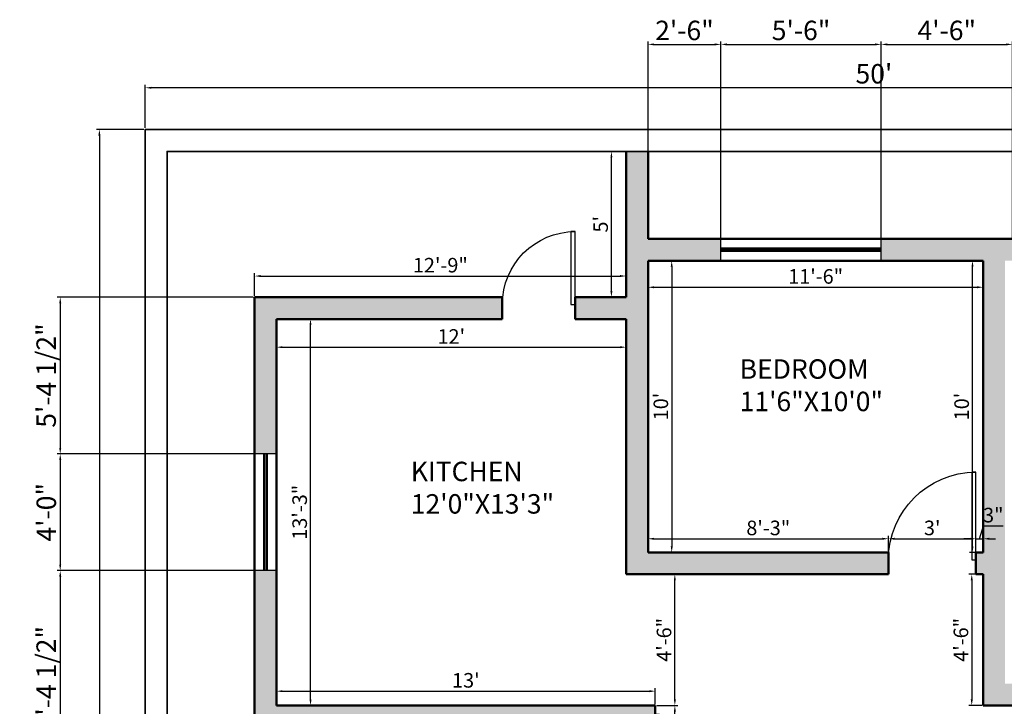
# Model space of a CAD drawing. Units: inches. Extents: x 2442 to 3851, y 589 to 2836.
# Tile 15 of 22: x 2442 to 2847, y 2554 to 2836. Entities that reach past the tile are written whole.
import ezdxf

# ---------------------------------------------------------------- set-up
doc = ezdxf.new("R2010")
doc.units = ezdxf.units.IN
for name, color, linetype, lineweight in [('A-ANNO-DIMS', 2, 'Continuous', 18), ('A-AREA-IDEN', 7, 'Continuous', 18), ('A-DOOR', 4, 'Continuous', 25), ('A-GLAZ', 1, 'Continuous', 25), ('A-WALL', 7, 'Continuous', 50), ('A-WALL-PATT', 8, 'Continuous', 13), ('C-PROP', 7, 'Continuous', 35)]:
    doc.layers.add(name, color=color, linetype=linetype, lineweight=lineweight)
doc.styles.get("Standard").update_dxf_attribs({"font": 'arial.ttf'})
doc.dimstyles.new('ISO-25', dxfattribs={"dimtxt": 8, "dimasz": 2.5, "dimexe": 1.25, "dimexo": 0.625, "dimtad": 1, "dimlunit": 3, "dimtxsty": 'Standard', "dimcen": 2.5, "dimadec": 0, "dimazin": 0, "dimtfac": 1, "dimtmove": 0, "dimatfit": 3, "dimfxl": 1, "dimarcsym": 0})

# ---------------------------------------------------------------- blocks, each defined once
blk = doc.blocks.new('*U23')
for p, q in [((0, 0), (0, -6)), ((36, 0), (36, -6))]:
    blk.add_line(p, q)
blk.add_lwpolyline([(0, 0), (0, 36), (1.75, 36), (1.75, 0)], close=True)
blk.add_arc((0, 0), 36, 0, 90)
blk = doc.blocks.new('*U24')
for p, q in [((0, 0), (0, -6)), ((30, 0), (30, -6))]:
    blk.add_line(p, q)
blk.add_lwpolyline([(0, 0), (0, 30), (1.75, 30), (1.75, 0)], close=True)
blk.add_arc((0, 0), 30, 0, 90)
blk = doc.blocks.new('*D35')
at = {"layer": 'A-ANNO-DIMS', "color": 0, "lineweight": -2, "transparency": 16777216}
for p, q in [((2493.6, 2791.83), (2493.6, 2809.62)), ((3093.6, 2791.83), (3093.6, 2809.62)), ((3091.1, 2808.37), (2496.1, 2808.37))]:
    blk.add_line(p, q, dxfattribs=at)
at = {"layer": 'A-ANNO-DIMS', "color": 0, "transparency": 16777216}
for points in [[(2496.1, 2808.78), (2496.1, 2807.95), (2493.6, 2808.37)], [(3091.1, 2808.78), (3091.1, 2807.95), (3093.6, 2808.37)]]:
    blk.add_solid(points, dxfattribs=at)
at = {"layer": 'Defpoints', "color": 0, "transparency": 16777216}
for p in [(2493.6, 2808.37), (2493.6, 2791.21), (3093.6, 2791.21)]:
    blk.add_point(p, dxfattribs=at)
at = {"layer": 'A-ANNO-DIMS', "color": 0, "transparency": 16777216, "insert": (2793.6, 2813.08), "char_height": 8, "attachment_point": 5}
blk.add_mtext("50'", dxfattribs=at)
blk = doc.blocks.new('*D36')
at = {"layer": 'A-ANNO-DIMS', "color": 0, "lineweight": -2, "transparency": 16777216}
for p, q in [((2492.97, 2791.21), (2473.47, 2791.21)), ((2474.72, 2788.71), (2474.72, 2193.71)), ((2492.97, 2191.21), (2473.47, 2191.21))]:
    blk.add_line(p, q, dxfattribs=at)
at = {"layer": 'A-ANNO-DIMS', "color": 0, "transparency": 16777216}
for points in [[(2474.3, 2788.71), (2475.14, 2788.71), (2474.72, 2791.21)], [(2474.3, 2193.71), (2475.14, 2193.71), (2474.72, 2191.21)]]:
    blk.add_solid(points, dxfattribs=at)
at = {"layer": 'Defpoints', "color": 0, "transparency": 16777216}
for p in [(2493.6, 2791.21), (2474.72, 2191.21), (2493.6, 2191.21)]:
    blk.add_point(p, dxfattribs=at)
at = {"layer": 'A-ANNO-DIMS', "color": 0, "transparency": 16777216, "insert": (2470.01, 2491.21), "char_height": 8, "attachment_point": 5, "rotation": 90}
blk.add_mtext("50'", dxfattribs=at)
blk = doc.blocks.new('*D37')
at = {"layer": 'A-ANNO-DIMS', "color": 0, "lineweight": -2, "transparency": 16777216}
for p, q in [((2548.22, 2713.21), (2562.89, 2713.21)), ((2561.64, 2556.71), (2561.64, 2710.71)), ((2548.22, 2554.21), (2562.89, 2554.21))]:
    blk.add_line(p, q, dxfattribs=at)
at = {"layer": 'A-ANNO-DIMS', "color": 0, "transparency": 16777216}
for points in [[(2561.22, 2710.71), (2562.05, 2710.71), (2561.64, 2713.21)], [(2561.22, 2556.71), (2562.05, 2556.71), (2561.64, 2554.21)]]:
    blk.add_solid(points, dxfattribs=at)
at = {"layer": 'Defpoints', "color": 0, "transparency": 16777216}
for p in [(2547.6, 2713.21), (2561.64, 2713.21), (2547.6, 2554.21)]:
    blk.add_point(p, dxfattribs=at)
at = {"layer": 'A-ANNO-DIMS', "color": 0, "transparency": 16777216, "insert": (2557.95, 2633.71), "char_height": 6, "attachment_point": 5, "rotation": 90}
blk.add_mtext('13\'-3"', dxfattribs=at)
blk = doc.blocks.new('*D38')
at = {"layer": 'A-ANNO-DIMS', "color": 0, "lineweight": -2, "transparency": 16777216}
for p, q in [((2547.6, 2712.58), (2547.6, 2700.38)), ((2691.6, 2712.58), (2691.6, 2700.38)), ((2550.1, 2701.63), (2689.1, 2701.63))]:
    blk.add_line(p, q, dxfattribs=at)
at = {"layer": 'A-ANNO-DIMS', "color": 0, "transparency": 16777216}
for points in [[(2550.1, 2702.05), (2550.1, 2701.22), (2547.6, 2701.63)], [(2689.1, 2702.05), (2689.1, 2701.22), (2691.6, 2701.63)]]:
    blk.add_solid(points, dxfattribs=at)
at = {"layer": 'Defpoints', "color": 0, "transparency": 16777216}
for p in [(2547.6, 2713.21), (2691.6, 2713.21), (2691.6, 2701.63)]:
    blk.add_point(p, dxfattribs=at)
at = {"layer": 'A-ANNO-DIMS', "color": 0, "transparency": 16777216, "insert": (2619.6, 2705.27), "char_height": 6, "attachment_point": 5}
blk.add_mtext("12'", dxfattribs=at)
blk = doc.blocks.new('*D39')
at = {"layer": 'A-ANNO-DIMS', "color": 0, "lineweight": -2, "transparency": 16777216}
for p, q in [((2690.97, 2782.21), (2684.27, 2782.21)), ((2685.52, 2724.71), (2685.52, 2779.71)), ((2690.97, 2722.21), (2684.27, 2722.21))]:
    blk.add_line(p, q, dxfattribs=at)
at = {"layer": 'A-ANNO-DIMS', "color": 0, "transparency": 16777216}
for points in [[(2685.11, 2779.71), (2685.94, 2779.71), (2685.52, 2782.21)], [(2685.11, 2724.71), (2685.94, 2724.71), (2685.52, 2722.21)]]:
    blk.add_solid(points, dxfattribs=at)
at = {"layer": 'Defpoints', "color": 0, "transparency": 16777216}
for p in [(2685.52, 2782.21), (2691.6, 2782.21), (2691.6, 2722.21)]:
    blk.add_point(p, dxfattribs=at)
at = {"layer": 'A-ANNO-DIMS', "color": 0, "transparency": 16777216, "insert": (2681.85, 2752.21), "char_height": 6, "attachment_point": 5, "rotation": 90}
blk.add_mtext("5'", dxfattribs=at)
blk = doc.blocks.new('*D40')
at = {"layer": 'A-ANNO-DIMS', "color": 0, "lineweight": -2, "transparency": 16777216}
for p, q in [((2538.6, 2722.83), (2538.6, 2732.15)), ((2541.1, 2730.9), (2689.1, 2730.9)), ((2691.6, 2722.83), (2691.6, 2732.15))]:
    blk.add_line(p, q, dxfattribs=at)
at = {"layer": 'A-ANNO-DIMS', "color": 0, "transparency": 16777216}
for points in [[(2541.1, 2731.32), (2541.1, 2730.49), (2538.6, 2730.9)], [(2689.1, 2731.32), (2689.1, 2730.49), (2691.6, 2730.9)]]:
    blk.add_solid(points, dxfattribs=at)
at = {"layer": 'Defpoints', "color": 0, "transparency": 16777216}
for p in [(2691.6, 2730.9), (2538.6, 2722.21), (2691.6, 2722.21)]:
    blk.add_point(p, dxfattribs=at)
at = {"layer": 'A-ANNO-DIMS', "color": 0, "transparency": 16777216, "insert": (2615.1, 2734.59), "char_height": 6, "attachment_point": 5}
blk.add_mtext('12\'-9"', dxfattribs=at)
blk = doc.blocks.new('*D44')
at = {"layer": 'A-ANNO-DIMS', "color": 0, "lineweight": -2, "transparency": 16777216}
for p, q in [((2700.6, 2736.58), (2700.6, 2725.04)), ((2838.6, 2736.58), (2838.6, 2725.04)), ((2703.1, 2726.29), (2836.1, 2726.29))]:
    blk.add_line(p, q, dxfattribs=at)
at = {"layer": 'A-ANNO-DIMS', "color": 0, "transparency": 16777216}
for points in [[(2703.1, 2726.7), (2703.1, 2725.87), (2700.6, 2726.29)], [(2836.1, 2726.7), (2836.1, 2725.87), (2838.6, 2726.29)]]:
    blk.add_solid(points, dxfattribs=at)
at = {"layer": 'Defpoints', "color": 0, "transparency": 16777216}
for p in [(2700.6, 2737.21), (2838.6, 2737.21), (2838.6, 2726.29)]:
    blk.add_point(p, dxfattribs=at)
at = {"layer": 'A-ANNO-DIMS', "color": 0, "transparency": 16777216, "insert": (2769.6, 2729.98), "char_height": 6, "attachment_point": 5}
blk.add_mtext('11\'-6"', dxfattribs=at)
blk = doc.blocks.new('*D45')
at = {"layer": 'A-ANNO-DIMS', "color": 0, "lineweight": -2, "transparency": 16777216}
for p, q in [((2701.22, 2737.21), (2711.59, 2737.21)), ((2710.34, 2734.71), (2710.34, 2619.71)), ((2701.22, 2617.21), (2711.59, 2617.21))]:
    blk.add_line(p, q, dxfattribs=at)
at = {"layer": 'A-ANNO-DIMS', "color": 0, "transparency": 16777216}
for points in [[(2709.93, 2734.71), (2710.76, 2734.71), (2710.34, 2737.21)], [(2709.93, 2619.71), (2710.76, 2619.71), (2710.34, 2617.21)]]:
    blk.add_solid(points, dxfattribs=at)
at = {"layer": 'Defpoints', "color": 0, "transparency": 16777216}
for p in [(2700.6, 2737.21), (2700.6, 2617.21), (2710.34, 2617.21)]:
    blk.add_point(p, dxfattribs=at)
at = {"layer": 'A-ANNO-DIMS', "color": 0, "transparency": 16777216, "insert": (2706.65, 2677.21), "char_height": 6, "attachment_point": 5, "rotation": 90}
blk.add_mtext("10'", dxfattribs=at)
blk = doc.blocks.new('*D60')
at = {"layer": 'A-ANNO-DIMS', "color": 0, "lineweight": -2, "transparency": 16777216}
for p, q in [((2837.97, 2737.21), (2832.93, 2737.21)), ((2834.18, 2619.71), (2834.18, 2734.71)), ((2837.97, 2617.21), (2832.93, 2617.21))]:
    blk.add_line(p, q, dxfattribs=at)
at = {"layer": 'A-ANNO-DIMS', "color": 0, "transparency": 16777216}
for points in [[(2833.76, 2734.71), (2834.6, 2734.71), (2834.18, 2737.21)], [(2833.76, 2619.71), (2834.6, 2619.71), (2834.18, 2617.21)]]:
    blk.add_solid(points, dxfattribs=at)
at = {"layer": 'Defpoints', "color": 0, "transparency": 16777216}
for p in [(2834.18, 2737.21), (2838.6, 2737.21), (2838.6, 2617.21)]:
    blk.add_point(p, dxfattribs=at)
at = {"layer": 'A-ANNO-DIMS', "color": 0, "transparency": 16777216, "insert": (2830.49, 2677.21), "char_height": 6, "attachment_point": 5, "rotation": 90}
blk.add_mtext("10'", dxfattribs=at)
blk = doc.blocks.new('*D61')
at = {"layer": 'A-ANNO-DIMS', "color": 0, "lineweight": -2, "transparency": 16777216}
for p, q in [((2700.6, 2617.83), (2700.6, 2624.06)), ((2703.1, 2622.81), (2797.1, 2622.81)), ((2799.6, 2617.83), (2799.6, 2624.06))]:
    blk.add_line(p, q, dxfattribs=at)
at = {"layer": 'A-ANNO-DIMS', "color": 0, "transparency": 16777216}
for points in [[(2703.1, 2623.23), (2703.1, 2622.4), (2700.6, 2622.81)], [(2797.1, 2623.23), (2797.1, 2622.4), (2799.6, 2622.81)]]:
    blk.add_solid(points, dxfattribs=at)
at = {"layer": 'Defpoints', "color": 0, "transparency": 16777216}
for p in [(2799.6, 2622.81), (2700.6, 2617.21), (2799.6, 2617.21)]:
    blk.add_point(p, dxfattribs=at)
at = {"layer": 'A-ANNO-DIMS', "color": 0, "transparency": 16777216, "insert": (2750.1, 2626.5), "char_height": 6, "attachment_point": 5}
blk.add_mtext('8\'-3"', dxfattribs=at)
blk = doc.blocks.new('*D62')
at = {"layer": 'A-ANNO-DIMS', "color": 0, "lineweight": -2, "transparency": 16777216}
for p, q in [((2799.6, 2617.83), (2799.6, 2624.06)), ((2802.1, 2622.81), (2833.1, 2622.81)), ((2835.6, 2614.83), (2835.6, 2624.06))]:
    blk.add_line(p, q, dxfattribs=at)
at = {"layer": 'A-ANNO-DIMS', "color": 0, "transparency": 16777216}
for points in [[(2802.1, 2623.23), (2802.1, 2622.4), (2799.6, 2622.81)], [(2833.1, 2623.23), (2833.1, 2622.4), (2835.6, 2622.81)]]:
    blk.add_solid(points, dxfattribs=at)
at = {"layer": 'Defpoints', "color": 0, "transparency": 16777216}
for p in [(2835.6, 2622.81), (2799.6, 2617.21), (2835.6, 2614.21)]:
    blk.add_point(p, dxfattribs=at)
at = {"layer": 'A-ANNO-DIMS', "color": 0, "transparency": 16777216, "insert": (2817.6, 2626.5), "char_height": 6, "attachment_point": 5}
blk.add_mtext("3'", dxfattribs=at)
blk = doc.blocks.new('*D63')
at = {"layer": 'A-ANNO-DIMS', "color": 0, "lineweight": -2, "transparency": 16777216}
for p, q in [((2837.1, 2622.81), (2838.67, 2628.07)), ((2838.67, 2628.07), (2846.82, 2628.07)), ((2833.1, 2622.81), (2830.6, 2622.81)), ((2835.6, 2614.83), (2835.6, 2624.06)), ((2835.6, 2622.81), (2838.6, 2622.81)), ((2835.6, 2622.81), (2838.6, 2622.81)), ((2838.6, 2617.83), (2838.6, 2624.06)), ((2841.1, 2622.81), (2843.6, 2622.81))]:
    blk.add_line(p, q, dxfattribs=at)
at = {"layer": 'A-ANNO-DIMS', "color": 0, "transparency": 16777216}
for points in [[(2833.1, 2623.23), (2833.1, 2622.4), (2835.6, 2622.81)], [(2841.1, 2623.23), (2841.1, 2622.4), (2838.6, 2622.81)]]:
    blk.add_solid(points, dxfattribs=at)
at = {"layer": 'Defpoints', "color": 0, "transparency": 16777216}
for p in [(2838.6, 2622.81), (2838.6, 2617.21), (2835.6, 2614.21)]:
    blk.add_point(p, dxfattribs=at)
at = {"layer": 'A-ANNO-DIMS', "color": 0, "transparency": 16777216, "insert": (2842.75, 2631.76), "char_height": 6, "attachment_point": 5}
blk.add_mtext('3"', dxfattribs=at)
blk = doc.blocks.new('*D85')
at = {"layer": 'A-ANNO-DIMS', "color": 0, "lineweight": -2, "transparency": 16777216}
for p, q in [((2704.22, 2554.21), (2712.89, 2554.21)), ((2711.64, 2544.71), (2711.64, 2551.71)), ((2704.22, 2542.21), (2712.89, 2542.21))]:
    blk.add_line(p, q, dxfattribs=at)
at = {"layer": 'A-ANNO-DIMS', "color": 0, "transparency": 16777216}
for points in [[(2711.22, 2551.71), (2712.05, 2551.71), (2711.64, 2554.21)], [(2711.22, 2544.71), (2712.05, 2544.71), (2711.64, 2542.21)]]:
    blk.add_solid(points, dxfattribs=at)
at = {"layer": 'Defpoints', "color": 0, "transparency": 16777216}
for p in [(2703.6, 2554.21), (2711.64, 2554.21), (2703.6, 2542.21)]:
    blk.add_point(p, dxfattribs=at)
at = {"layer": 'A-ANNO-DIMS', "color": 0, "transparency": 16777216, "insert": (2708, 2548.21), "char_height": 6, "attachment_point": 5, "rotation": 90}
blk.add_mtext("1'", dxfattribs=at)
blk = doc.blocks.new('*D86')
at = {"layer": 'A-ANNO-DIMS', "color": 0, "lineweight": -2, "transparency": 16777216}
for p, q in [((2709.79, 2608.21), (2712.89, 2608.21)), ((2711.64, 2556.71), (2711.64, 2605.71)), ((2704.22, 2554.21), (2712.89, 2554.21))]:
    blk.add_line(p, q, dxfattribs=at)
at = {"layer": 'A-ANNO-DIMS', "color": 0, "transparency": 16777216}
for points in [[(2711.22, 2605.71), (2712.05, 2605.71), (2711.64, 2608.21)], [(2711.22, 2556.71), (2712.05, 2556.71), (2711.64, 2554.21)]]:
    blk.add_solid(points, dxfattribs=at)
at = {"layer": 'Defpoints', "color": 0, "transparency": 16777216}
for p in [(2709.17, 2608.21), (2711.64, 2608.21), (2703.6, 2554.21)]:
    blk.add_point(p, dxfattribs=at)
at = {"layer": 'A-ANNO-DIMS', "color": 0, "transparency": 16777216, "insert": (2707.95, 2581.21), "char_height": 6, "attachment_point": 5, "rotation": 90}
blk.add_mtext('4\'-6"', dxfattribs=at)
blk = doc.blocks.new('*D87')
at = {"layer": 'A-ANNO-DIMS', "color": 0, "lineweight": -2, "transparency": 16777216}
for p, q in [((2837.97, 2608.21), (2832.63, 2608.21)), ((2833.88, 2605.71), (2833.88, 2556.71)), ((2837.97, 2554.21), (2832.63, 2554.21))]:
    blk.add_line(p, q, dxfattribs=at)
at = {"layer": 'A-ANNO-DIMS', "color": 0, "transparency": 16777216}
for points in [[(2833.46, 2605.71), (2834.29, 2605.71), (2833.88, 2608.21)], [(2833.46, 2556.71), (2834.29, 2556.71), (2833.88, 2554.21)]]:
    blk.add_solid(points, dxfattribs=at)
at = {"layer": 'Defpoints', "color": 0, "transparency": 16777216}
for p in [(2838.6, 2608.21), (2833.88, 2554.21), (2838.6, 2554.21)]:
    blk.add_point(p, dxfattribs=at)
at = {"layer": 'A-ANNO-DIMS', "color": 0, "transparency": 16777216, "insert": (2830.19, 2581.21), "char_height": 6, "attachment_point": 5, "rotation": 90}
blk.add_mtext('4\'-6"', dxfattribs=at)
blk = doc.blocks.new('*D88')
at = {"layer": 'A-ANNO-DIMS', "color": 0, "lineweight": -2, "transparency": 16777216}
for p, q in [((2547.6, 2554.83), (2547.6, 2561.35)), ((2550.1, 2560.1), (2701.1, 2560.1)), ((2703.6, 2554.83), (2703.6, 2561.35))]:
    blk.add_line(p, q, dxfattribs=at)
at = {"layer": 'A-ANNO-DIMS', "color": 0, "transparency": 16777216}
for points in [[(2550.1, 2560.52), (2550.1, 2559.68), (2547.6, 2560.1)], [(2701.1, 2560.52), (2701.1, 2559.68), (2703.6, 2560.1)]]:
    blk.add_solid(points, dxfattribs=at)
at = {"layer": 'Defpoints', "color": 0, "transparency": 16777216}
for p in [(2703.6, 2560.1), (2547.6, 2554.21), (2703.6, 2554.21)]:
    blk.add_point(p, dxfattribs=at)
at = {"layer": 'A-ANNO-DIMS', "color": 0, "transparency": 16777216, "insert": (2625.6, 2563.79), "char_height": 6, "attachment_point": 5}
blk.add_mtext("13'", dxfattribs=at)
blk = doc.blocks.new('*D182')
at = {"layer": 'A-ANNO-DIMS', "color": 0, "lineweight": -2, "transparency": 16777216}
for p, q in [((2700.6, 2746.83), (2700.6, 2827.46)), ((2703.1, 2826.21), (2728.1, 2826.21)), ((2730.6, 2746.83), (2730.6, 2827.46))]:
    blk.add_line(p, q, dxfattribs=at)
at = {"layer": 'A-ANNO-DIMS', "color": 0, "transparency": 16777216}
for points in [[(2703.1, 2826.62), (2703.1, 2825.79), (2700.6, 2826.21)], [(2728.1, 2826.62), (2728.1, 2825.79), (2730.6, 2826.21)]]:
    blk.add_solid(points, dxfattribs=at)
at = {"layer": 'Defpoints', "color": 0, "transparency": 16777216}
for p in [(2730.6, 2826.21), (2700.6, 2746.21), (2730.6, 2746.21)]:
    blk.add_point(p, dxfattribs=at)
at = {"layer": 'A-ANNO-DIMS', "color": 0, "transparency": 16777216, "insert": (2715.6, 2830.92), "char_height": 8, "attachment_point": 5}
blk.add_mtext('2\'-6"', dxfattribs=at)
blk = doc.blocks.new('*D183')
at = {"layer": 'A-ANNO-DIMS', "color": 0, "lineweight": -2, "transparency": 16777216}
for p, q in [((2730.6, 2746.83), (2730.6, 2827.46)), ((2733.1, 2826.21), (2794.1, 2826.21)), ((2796.6, 2746.83), (2796.6, 2827.46))]:
    blk.add_line(p, q, dxfattribs=at)
at = {"layer": 'A-ANNO-DIMS', "color": 0, "transparency": 16777216}
for points in [[(2733.1, 2826.62), (2733.1, 2825.79), (2730.6, 2826.21)], [(2794.1, 2826.62), (2794.1, 2825.79), (2796.6, 2826.21)]]:
    blk.add_solid(points, dxfattribs=at)
at = {"layer": 'Defpoints', "color": 0, "transparency": 16777216}
for p in [(2796.6, 2826.21), (2730.6, 2746.21), (2796.6, 2746.21)]:
    blk.add_point(p, dxfattribs=at)
at = {"layer": 'A-ANNO-DIMS', "color": 0, "transparency": 16777216, "insert": (2763.6, 2830.92), "char_height": 8, "attachment_point": 5}
blk.add_mtext('5\'-6"', dxfattribs=at)
blk = doc.blocks.new('*D184')
at = {"layer": 'A-ANNO-DIMS', "color": 0, "lineweight": -2, "transparency": 16777216}
for p, q in [((2796.6, 2746.83), (2796.6, 2827.46)), ((2799.1, 2826.21), (2848.1, 2826.21)), ((2850.6, 2746.83), (2850.6, 2827.46))]:
    blk.add_line(p, q, dxfattribs=at)
at = {"layer": 'A-ANNO-DIMS', "color": 0, "transparency": 16777216}
for points in [[(2799.1, 2826.62), (2799.1, 2825.79), (2796.6, 2826.21)], [(2848.1, 2826.62), (2848.1, 2825.79), (2850.6, 2826.21)]]:
    blk.add_solid(points, dxfattribs=at)
at = {"layer": 'Defpoints', "color": 0, "transparency": 16777216}
for p in [(2850.6, 2826.21), (2796.6, 2746.21), (2850.6, 2746.21)]:
    blk.add_point(p, dxfattribs=at)
at = {"layer": 'A-ANNO-DIMS', "color": 0, "transparency": 16777216, "insert": (2823.6, 2830.92), "char_height": 8, "attachment_point": 5}
blk.add_mtext('4\'-6"', dxfattribs=at)
blk = doc.blocks.new('*D198')
at = {"layer": 'A-ANNO-DIMS', "color": 0, "lineweight": -2, "transparency": 16777216}
for p, q in [((2537.97, 2722.21), (2457.35, 2722.21)), ((2458.6, 2719.71), (2458.6, 2660.21)), ((2537.97, 2657.71), (2457.35, 2657.71))]:
    blk.add_line(p, q, dxfattribs=at)
at = {"layer": 'A-ANNO-DIMS', "color": 0, "transparency": 16777216}
for points in [[(2458.18, 2719.71), (2459.02, 2719.71), (2458.6, 2722.21)], [(2458.18, 2660.21), (2459.02, 2660.21), (2458.6, 2657.71)]]:
    blk.add_solid(points, dxfattribs=at)
at = {"layer": 'Defpoints', "color": 0, "transparency": 16777216}
for p in [(2538.6, 2722.21), (2458.6, 2657.71), (2538.6, 2657.71)]:
    blk.add_point(p, dxfattribs=at)
at = {"layer": 'A-ANNO-DIMS', "color": 0, "transparency": 16777216, "insert": (2453.84, 2689.96), "char_height": 8, "attachment_point": 5, "rotation": 90}
blk.add_mtext('5\'-4 1/2"', dxfattribs=at)
blk = doc.blocks.new('*D199')
at = {"layer": 'A-ANNO-DIMS', "color": 0, "lineweight": -2, "transparency": 16777216}
for p, q in [((2537.97, 2657.71), (2457.35, 2657.71)), ((2458.6, 2655.21), (2458.6, 2612.21)), ((2537.97, 2609.71), (2457.35, 2609.71))]:
    blk.add_line(p, q, dxfattribs=at)
at = {"layer": 'A-ANNO-DIMS', "color": 0, "transparency": 16777216}
for points in [[(2458.18, 2655.21), (2459.02, 2655.21), (2458.6, 2657.71)], [(2458.18, 2612.21), (2459.02, 2612.21), (2458.6, 2609.71)]]:
    blk.add_solid(points, dxfattribs=at)
at = {"layer": 'Defpoints', "color": 0, "transparency": 16777216}
for p in [(2538.6, 2657.71), (2458.6, 2609.71), (2538.6, 2609.71)]:
    blk.add_point(p, dxfattribs=at)
at = {"layer": 'A-ANNO-DIMS', "color": 0, "transparency": 16777216, "insert": (2453.89, 2633.71), "char_height": 8, "attachment_point": 5, "rotation": 90}
blk.add_mtext('4\'-0"', dxfattribs=at)
blk = doc.blocks.new('*D200')
at = {"layer": 'A-ANNO-DIMS', "color": 0, "lineweight": -2, "transparency": 16777216}
for p, q in [((2537.97, 2609.71), (2457.35, 2609.71)), ((2458.6, 2607.21), (2458.6, 2523.71)), ((2537.97, 2521.21), (2457.35, 2521.21))]:
    blk.add_line(p, q, dxfattribs=at)
at = {"layer": 'A-ANNO-DIMS', "color": 0, "transparency": 16777216}
for points in [[(2458.18, 2607.21), (2459.02, 2607.21), (2458.6, 2609.71)], [(2458.18, 2523.71), (2459.02, 2523.71), (2458.6, 2521.21)]]:
    blk.add_solid(points, dxfattribs=at)
at = {"layer": 'Defpoints', "color": 0, "transparency": 16777216}
for p in [(2538.6, 2609.71), (2458.6, 2521.21), (2538.6, 2521.21)]:
    blk.add_point(p, dxfattribs=at)
at = {"layer": 'A-ANNO-DIMS', "color": 0, "transparency": 16777216, "insert": (2453.84, 2565.46), "char_height": 8, "attachment_point": 5, "rotation": 90}
blk.add_mtext('7\'-4 1/2"', dxfattribs=at)

msp = doc.modelspace()

# ---------------------------------------------------------------- hatches: boundary and pattern name
at = {"layer": 'A-WALL-PATT'}
h = msp.add_hatch(color=256, dxfattribs=at)
h.dxf.hatch_style = 1
h.paths.add_polyline_path([(2640.599, 2713.208), (2640.599, 2719.208), (2640.599, 2722.208), (2538.599, 2722.208), (2538.599, 2657.708), (2547.599, 2657.708), (2547.599, 2713.208)])
h.paths.add_polyline_path([(2700.599, 2737.208), (2730.599, 2737.208), (2730.599, 2746.208), (2700.599, 2746.208), (2700.599, 2782.208), (2691.599, 2782.208), (2691.599, 2722.208), (2670.599, 2722.208), (2670.599, 2719.208), (2670.599, 2713.208), (2691.599, 2713.208), (2691.599, 2608.208), (2799.599, 2608.208), (2799.599, 2614.208), (2799.599, 2617.208), (2700.599, 2617.208)])
h.paths.add_polyline_path([(2838.599, 2737.208), (2838.599, 2617.208), (2835.599, 2617.208), (2835.599, 2614.208), (2835.599, 2608.208), (2838.599, 2608.208), (2838.599, 2554.208), (2850.599, 2554.208), (2850.599, 2560.208), (2850.599, 2563.208), (2847.599, 2563.208), (2847.599, 2737.208), (2850.599, 2737.208), (2850.599, 2746.208), (2796.599, 2746.208), (2796.599, 2737.208)])
h.paths.add_polyline_path([(2898.599, 2746.208), (2898.599, 2737.208), (2967.599, 2737.208), (2967.599, 2746.208)])
h.paths.add_polyline_path([(3048.599, 2746.208), (3015.599, 2746.208), (3015.599, 2737.208), (3039.599, 2737.208), (3039.599, 2665.208), (3048.599, 2665.208)])
h.paths.add_polyline_path([(3039.599, 2611.208), (3039.599, 2605.208), (3048.599, 2605.208), (3048.599, 2617.208), (2946.599, 2617.208), (2946.599, 2611.208)])
h.paths.add_polyline_path([(2961.599, 2563.208), (2961.599, 2581.208), (2955.599, 2581.208), (2955.599, 2563.208), (2895.599, 2563.208), (2895.599, 2611.208), (2916.599, 2611.208), (2916.599, 2617.208), (2889.599, 2617.208), (2889.599, 2563.208), (2886.599, 2563.208), (2886.599, 2554.208), (2937.599, 2554.208), (2937.599, 2536.208), (2943.599, 2536.208), (2943.599, 2554.208), (3039.599, 2554.208), (3039.599, 2548.208), (3048.599, 2548.208), (3048.599, 2569.208), (3039.599, 2569.208), (3039.599, 2563.208)])
h.paths.add_polyline_path([(2538.599, 2521.208), (2547.599, 2521.208), (2547.599, 2545.208), (2694.599, 2545.208), (2694.599, 2542.208), (2697.599, 2542.208), (2703.599, 2542.208), (2703.599, 2554.208), (2547.599, 2554.208), (2547.599, 2609.708), (2538.599, 2609.708)])
h.paths.add_polyline_path([(2538.599, 2368.208), (2547.599, 2368.208), (2547.599, 2392.208), (2694.599, 2392.208), (2694.599, 2344.208), (2703.599, 2344.208), (2703.599, 2506.208), (2697.599, 2506.208), (2694.599, 2506.208), (2694.599, 2401.208), (2547.599, 2401.208), (2547.599, 2473.208), (2538.599, 2473.208)])
h.paths.add_polyline_path([(2547.599, 2287.208), (2553.599, 2287.208), (2553.599, 2293.208), (2553.599, 2296.208), (2547.599, 2296.208), (2547.599, 2320.208), (2538.599, 2320.208), (2538.599, 2191.208), (2547.599, 2191.208)])
h.paths.add_polyline_path([(2703.599, 2296.208), (2670.599, 2296.208), (2670.599, 2287.208), (2694.599, 2287.208), (2694.599, 2248.208), (2733.599, 2248.208), (2733.599, 2257.208), (2703.599, 2257.208)])
h.paths.add_polyline_path([(2593.599, 2287.208), (2604.599, 2287.208), (2604.599, 2296.208), (2593.599, 2296.208)])
h.paths.add_polyline_path([(2799.599, 2248.208), (2799.599, 2257.208), (2775.599, 2257.208), (2775.599, 2248.208)])
h.paths.add_polyline_path([(2892.599, 2248.208), (2892.599, 2287.208), (2883.599, 2287.208), (2883.599, 2257.208), (2865.599, 2257.208), (2865.599, 2248.208)])
h.paths.add_polyline_path([(2883.599, 2353.208), (2892.599, 2353.208), (2892.599, 2392.208), (3048.599, 2392.208), (3048.599, 2426.708), (3039.599, 2426.708), (3039.599, 2401.208), (2892.599, 2401.208), (2892.599, 2461.208), (2883.599, 2461.208)])
h.paths.add_polyline_path([(3039.599, 2474.708), (3048.599, 2474.708), (3048.599, 2512.208), (3039.599, 2512.208), (3039.599, 2506.208), (2937.599, 2506.208), (2937.599, 2500.208), (3039.599, 2500.208)])

# ---------------------------------------------------------------- linework, layer by layer
at = {"layer": 'A-GLAZ'}
for p, q in [((2730.599, 2737.208), (2730.599, 2746.208)), ((2796.599, 2737.208), (2796.599, 2746.208)), ((2547.599, 2657.708), (2538.599, 2657.708)), ((2547.599, 2609.708), (2538.599, 2609.708))]:
    msp.add_line(p, q, dxfattribs=at)
at = {"layer": 'A-WALL'}
for p, q in [((2691.599, 2722.208), (2691.599, 2782.208)), ((2700.599, 2746.208), (2700.599, 2782.208)), ((2700.599, 2746.208), (3048.599, 2746.208)), ((2730.599, 2742.208), (2796.599, 2742.208)), ((2730.599, 2741.208), (2796.599, 2741.208)), ((2700.599, 2617.208), (2700.599, 2737.208)), ((2700.599, 2737.208), (2838.599, 2737.208)), ((2838.599, 2617.208), (2838.599, 2737.208)), ((2538.599, 2722.208), (2538.599, 2191.208)), ((2538.599, 2722.208), (2640.599, 2722.208)), ((2640.599, 2713.208), (2640.599, 2722.208)), ((2670.599, 2713.208), (2670.599, 2722.208)), ((2670.599, 2722.208), (2691.599, 2722.208)), ((2547.599, 2713.208), (2547.599, 2554.208)), ((2547.599, 2713.208), (2640.599, 2713.208)), ((2670.599, 2713.208), (2691.599, 2713.208)), ((2691.599, 2608.208), (2691.599, 2713.208)), ((2542.599, 2657.708), (2542.599, 2609.708)), ((2543.599, 2657.708), (2543.599, 2609.708)), ((2700.599, 2617.208), (2799.599, 2617.208)), ((2799.599, 2608.208), (2799.599, 2617.208)), ((2835.599, 2608.208), (2835.599, 2617.208)), ((2835.599, 2617.208), (2838.599, 2617.208)), ((2691.599, 2608.208), (2799.599, 2608.208)), ((2835.599, 2608.208), (2838.599, 2608.208)), ((2838.599, 2554.208), (2838.599, 2608.208)), ((2547.599, 2554.208), (2703.599, 2554.208)), ((2703.599, 2542.208), (2703.599, 2554.208)), ((2838.599, 2554.208), (2850.599, 2554.208))]:
    msp.add_line(p, q, dxfattribs=at)
at = {"layer": 'C-PROP'}
for points in [[(3066.599, 2191.208), (3093.599, 2191.208), (3093.599, 2791.208), (2493.599, 2791.208), (2493.599, 2191.208), (2738.599, 2191.208)], [(3066.599, 2200.208), (3084.599, 2200.208), (3084.599, 2782.208), (2502.599, 2782.208), (2502.599, 2200.208), (2538.599, 2200.208)]]:
    msp.add_lwpolyline(points, dxfattribs=at)

# ---------------------------------------------------------------- block references
at = {"layer": 'A-DOOR', "xscale": -1}
for name, p in [('*U24', (2670.599, 2719.208)), ('*U23', (2835.599, 2614.208))]:
    msp.add_blockref(name, p, dxfattribs=at)

# ---------------------------------------------------------------- texts
at = {"layer": 'A-AREA-IDEN', "char_height": 8, "attachment_point": 1}
for s, insert in [('{\\fTimes New Roman|b0|i0|c0|p18;BEDROOM\\P11\'6"X10\'0"}', (2738.331, 2696.643)), ('{\\fTimes New Roman|b0|i0|c0|p18;KITCHEN\\P12\'0"X13\'3"}', (2602.937, 2654.503))]:
    msp.add_mtext_dynamic_manual_height_columns(s, width=110.76054, gutter_width=12.5, heights=[0], dxfattribs=dict(at, insert=insert))

# ---------------------------------------------------------------- dimensions: what is measured, and where the dimension line sits
at = {"layer": 'A-ANNO-DIMS'}
for base, p1, p2, override, picture, middle in [((2730.599, 2826.208), (2700.599, 2746.208), (2730.599, 2746.208), {"dimdec": 1, "dimlfac": 1, "dimrnd": 0, "dimzin": 1, "dimdsep": 46, "dimlunit": 4, "dimfrac": 2}, '*D182', (2715.599, 2830.917)), ((2796.599, 2826.208), (2730.599, 2746.208), (2796.599, 2746.208), {"dimdec": 1, "dimlfac": 1, "dimrnd": 0, "dimzin": 1, "dimdsep": 46, "dimlunit": 4, "dimfrac": 2}, '*D183', (2763.599, 2830.917)), ((2850.599, 2826.208), (2796.599, 2746.208), (2850.599, 2746.208), {"dimdec": 1, "dimlfac": 1, "dimrnd": 0, "dimzin": 1, "dimdsep": 46, "dimlunit": 4, "dimfrac": 2}, '*D184', (2823.599, 2830.917)), ((2493.599, 2808.367), (3093.599, 2791.208), (2493.599, 2791.208), {"dimclrd": 0, "dimclre": 0, "dimclrt": 0}, '*D35', (2793.599, 2813.076)), ((2691.599, 2730.903), (2538.599, 2722.208), (2691.599, 2722.208), {"dimtxt": 6, "dimclrd": 0, "dimclre": 0, "dimclrt": 0}, '*D40', (2615.099, 2734.592)), ((2838.599, 2726.288), (2700.599, 2737.208), (2838.599, 2737.208), {"dimtxt": 6, "dimclrd": 0, "dimclre": 0, "dimclrt": 0}, '*D44', (2769.599, 2729.977)), ((2691.599, 2701.635), (2547.599, 2713.208), (2691.599, 2713.208), {"dimtxt": 6, "dimclrd": 0, "dimclre": 0, "dimclrt": 0}, '*D38', (2619.599, 2705.272)), ((2838.599, 2622.812), (2835.599, 2614.208), (2838.599, 2617.208), {"dimtxt": 6, "dimclrd": 0, "dimclre": 0, "dimclrt": 0, "dimtmove": 1}, '*D63', (2839.3, 2631.756)), ((2799.599, 2622.812), (2700.599, 2617.208), (2799.599, 2617.208), {"dimtxt": 6, "dimclrd": 0, "dimclre": 0, "dimclrt": 0}, '*D61', (2750.099, 2626.503)), ((2835.599, 2622.812), (2799.599, 2617.208), (2835.599, 2614.208), {"dimtxt": 6, "dimclrd": 0, "dimclre": 0, "dimclrt": 0, "dimtmove": 1}, '*D62', (2817.599, 2626.503)), ((2703.599, 2560.1), (2547.599, 2554.208), (2703.599, 2554.208), {"dimtxt": 6, "dimclrd": 0, "dimclre": 0, "dimclrt": 0}, '*D88', (2625.599, 2563.791))]:
    dim = msp.add_linear_dim(base=base, p1=p1, p2=p2, dimstyle='ISO-25', override=override, dxfattribs=at)
    dim.commit()
    dim.dimension.update_dxf_attribs({"geometry": picture, "text_midpoint": middle})
for base, p1, p2, angle, override, picture, middle in [((2474.719, 2191.208), (2493.599, 2791.208), (2493.599, 2191.208), 90, {"dimclrd": 0, "dimclre": 0, "dimclrt": 0}, '*D36', (2470.009, 2491.208)), ((2685.523, 2782.208), (2691.599, 2722.208), (2691.599, 2782.208), 90, {"dimtxt": 6, "dimclrd": 0, "dimclre": 0, "dimclrt": 0}, '*D39', (2681.847, 2752.208)), ((2710.342, 2617.208), (2700.599, 2737.208), (2700.599, 2617.208), 90, {"dimtxt": 6, "dimclrd": 0, "dimclre": 0, "dimclrt": 0}, '*D45', (2706.654, 2677.208)), ((2834.179, 2737.208), (2838.599, 2617.208), (2838.599, 2737.208), 90, {"dimtxt": 6, "dimclrd": 0, "dimclre": 0, "dimclrt": 0}, '*D60', (2830.491, 2677.208)), ((2458.599, 2657.708), (2538.599, 2722.208), (2538.599, 2657.708), 90, {"dimdec": 1, "dimlfac": 1, "dimrnd": 0, "dimzin": 1, "dimdsep": 46, "dimlunit": 4, "dimfrac": 2}, '*D198', (2453.837, 2689.958)), ((2561.637, 2713.208), (2547.599, 2554.208), (2547.599, 2713.208), 270, {"dimtxt": 6, "dimclrd": 0, "dimclre": 0, "dimclrt": 0}, '*D37', (2557.947, 2633.708)), ((2458.599, 2609.708), (2538.599, 2657.708), (2538.599, 2609.708), 90, {"dimdec": 1, "dimlfac": 1, "dimrnd": 0, "dimzin": 1, "dimdsep": 46, "dimlunit": 4, "dimfrac": 2}, '*D199', (2453.889, 2633.708)), ((2458.599, 2521.208), (2538.599, 2609.708), (2538.599, 2521.208), 90, {"dimdec": 1, "dimlfac": 1, "dimrnd": 0, "dimzin": 1, "dimdsep": 46, "dimlunit": 4, "dimfrac": 2}, '*D200', (2453.837, 2565.458)), ((2711.636, 2608.208), (2703.599, 2554.208), (2709.168, 2608.208), 90, {"dimtxt": 6, "dimclrd": 0, "dimclre": 0, "dimclrt": 0, "dimtmove": 1}, '*D86', (2707.947, 2581.208)), ((2833.875, 2554.208), (2838.599, 2608.208), (2838.599, 2554.208), 90, {"dimtxt": 6, "dimclrd": 0, "dimclre": 0, "dimclrt": 0}, '*D87', (2830.187, 2581.208)), ((2711.636, 2554.208), (2703.599, 2542.208), (2703.599, 2554.208), 90, {"dimtxt": 6, "dimclrd": 0, "dimclre": 0, "dimclrt": 0, "dimtmove": 1}, '*D85', (2707.998, 2548.208))]:
    dim = msp.add_linear_dim(base=base, p1=p1, p2=p2, angle=angle, dimstyle='ISO-25', override=override, dxfattribs=at)
    dim.commit()
    dim.dimension.update_dxf_attribs({"geometry": picture, "text_midpoint": middle})

doc.saveas('drawing.dxf')
